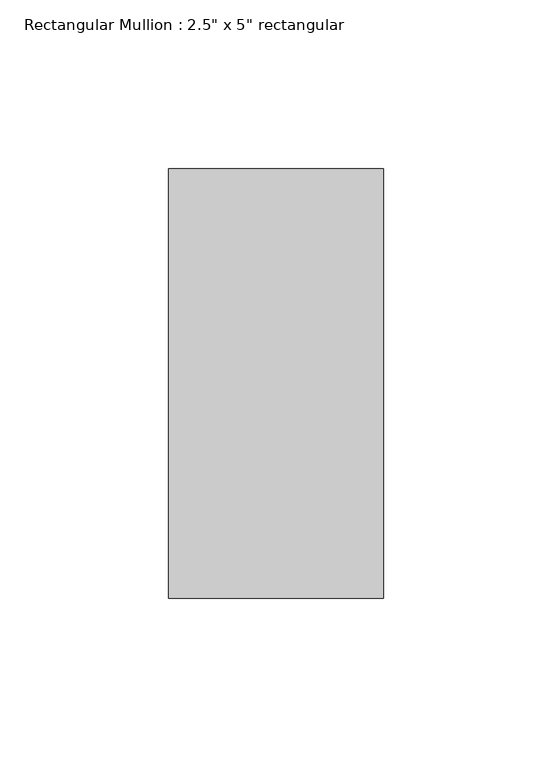
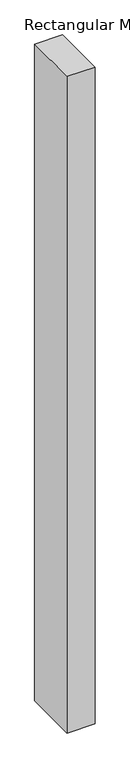
"""IFC4 building model written with IfcOpenShell, lengths in millimetres: member geometry."""

from ifc_helpers import new_model, si_unit, frame, origin, place, context, project, spatial, polyline, outline, extrude, source, transform, mapped, element, save


def member_69a5b808(model_context):
    return source(origin(), model_context, "Body", "SweptSolid", [
        extrude(outline(polyline([(31.75, 63.5), (31.75, -63.5), (-31.75, -63.5), (-31.75, 63.5), (31.75, 63.5)])), frame((0.0, 0.0, -1575.4674874), z_axis=(0.0, 0.0, 1.0), x_axis=(1.0, 0.0, 0.0)), (0.0, 0.0, 1.0), 1575.4674874),
    ])


if __name__ == "__main__":
    model = new_model("IFC4")
    model_context = context("Model", 3, world=origin())
    ifc_project = project(units=[si_unit("LENGTHUNIT", "METRE", prefix="MILLI")], contexts=[model_context])
    site = spatial("IfcSite", under=ifc_project)
    building = spatial("IfcBuilding", under=site)
    placement = place(None, origin())
    member_shape = member_69a5b808(model_context)
    element("IfcMember", 1, ObjectType="Rectangular Mullion : 2.5\" x 5\" rectangular", at=placement, inside=building, context=model_context, shape_type="MappedRepresentation", body=[
        mapped(member_shape, transform((0.0, 0.0, 0.0), x_axis=(1.0, 0.0, 0.0), y_axis=(0.0, 1.0, 0.0), z_axis=(0.0, 0.0, 1.0))),
    ])
    save(model, "model.ifc")

# Revit data of these elements
# Type "Rectangular Mullion : 2.5\" x 5\" rectangular"
#   built-in parameter 1007304 = 0.416667 (stored number, unit not read)
#   built-in parameter 1007301 = 0.104167 (stored number, unit not read)
#   built-in parameter 1007300 = 0.104167 (stored number, unit not read)
# Element 1 (IfcMember, "Rectangular Mullion : 2.5\" x 5\" rectangular")
#   Materials on its faces: "Aluminum"
# Materials
#   "Aluminum": class "Metal", colour RGB 247 247 247, transparency 0, Description = "Aluminum 6061", Cost = 0
